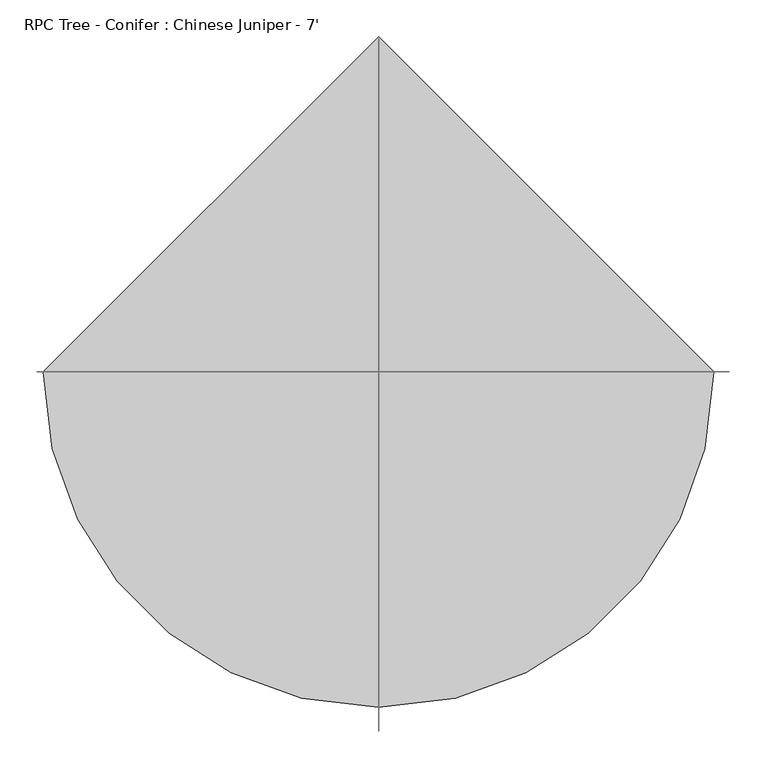
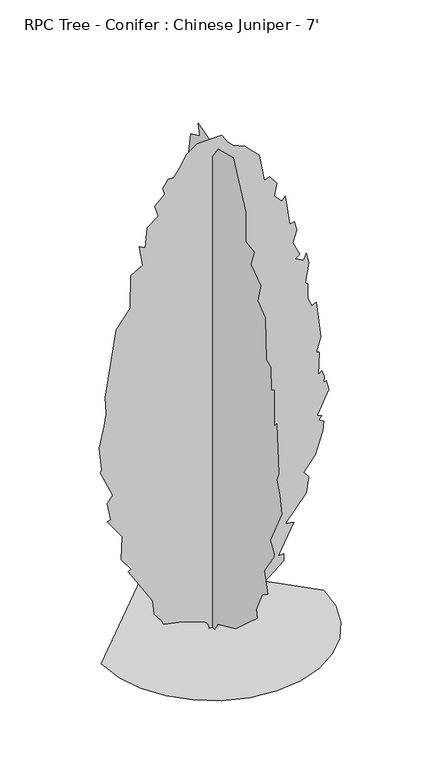
"""IFC4 building model written with IfcOpenShell, lengths in millimetres: geographic element geometry, RPC Tree - Conifer : Chinese Juniper - 7'."""

from ifc_helpers import new_model, si_unit, origin, place, context, project, spatial, triangles, source, transform, mapped, element, save


def rpc_tree_conifer_chinese_juniper_7_1b9786cd(model_context):
    return source(origin(), model_context, "Body", "Tessellation", [
        triangles([(-14.517647, 6e-07, 1.3e-06), (-18.0071097, -3e-07, 17.9396969), (-27.4223632, -6e-07, 30.3914521), (-123.5685295, 1.5e-06, 65.7757953), (-201.676062, 3.9e-06, 82.3498608), (-209.1624873, 3.1e-06, 101.0656516), (-239.326362, 2.1e-06, 139.6788561), (-246.5945957, -1e-06, 198.3880905), (-257.8249785, -1.9e-06, 220.8470939), (-347.6599566, -6.4e-06, 363.0865585), (-336.0369015, -7.4e-06, 370.071561), (-375.7854927, -8.9e-06, 425.7942498), (-371.7570322, -1.5e-05, 524.6285151), (-433.7535387, -1.74e-05, 610.1379032), (-418.7802157, -1.83e-05, 613.8793173), (-433.1718882, -2.22e-05, 689.5207758), (-411.2922644, -2.49e-05, 718.6876728), (-463.6977139, -2.95e-05, 834.7279736), (-456.2123059, -3.02e-05, 842.2133451), (-467.4416714, -3.58e-05, 943.2777431), (-447.126705, -4.19e-05, 1031.4541197), (-437.4949891, -4.53e-05, 1081.7767748), (-441.2389466, -4.94e-05, 1152.8969976), (-396.3214485, -6.81e-05, 1433.6338589), (-340.174585, -7.5e-05, 1508.4981846), (-337.1392688, -8.35e-05, 1648.2265743), (-287.7691355, -8.74e-05, 1676.941246), (-302.7424948, -9.18e-05, 1763.0323574), (-277.1874594, -9.21e-05, 1748.371479), (-269.0543621, -9.76e-05, 1834.1525803), (-224.1350836, -0.0001015, 1867.8406403), (-239.107916, -0.0001038, 1916.5022049), (-197.9328675, -0.0001078, 1953.9342224), (-205.4192747, -0.000109, 1980.1369835), (-182.9602713, -0.000112, 2013.8251888), (-160.5012679, -0.000113, 2013.8251888), (-134.7328734, -0.0001161, 2047.2821583), (-108.898967, -0.0001202, 2095.8470718), (-62.5486394, -0.0001241, 2127.2339642), (37.1144179, -0.0001285, 2128.801165), (60.3458442, -0.0001273, 2092.4307106), (82.8048476, -0.000127, 2069.9720524), (132.737601, -0.0001279, 2048.8239246), (191.3566519, -0.0001268, 1987.6224277), (213.8156735, -0.0001209, 1871.5845978), (236.2746769, -0.0001223, 1879.070042), (263.6666277, -0.0001212, 1839.8828991), (254.989959, -0.0001178, 1789.2351185), (284.9366594, -0.0001171, 1755.5469131), (299.9074571, -0.0001186, 1770.5202724), (318.6248102, -0.0001119, 1643.2505699), (337.3395836, -0.0001129, 1646.9946728), (347.517378, -0.0001111, 1609.9130699), (330.7888933, -0.0001074, 1559.0291119), (359.7983145, -0.000105, 1497.2687828), (340.1843954, -0.0001034, 1485.5084541), (374.7716738, -0.0001038, 1467.3220642), (386.0010392, -0.0001059, 1493.5248253), (397.230441, -0.0001037, 1448.6072182), (382.2596251, -9.81e-05, 1366.2577389), (393.0673594, -9.81e-05, 1357.3651131), (391.5662155, -9.44e-05, 1296.562429), (408.4598064, -9.28e-05, 1257.7053532), (427.1771233, -9.41e-05, 1265.1907974), (445.8918966, -8.55e-05, 1107.9794632), (427.1771233, -8.11e-05, 1048.0886421), (438.8332068, -8.14e-05, 1044.1287821), (434.6625312, -7.54e-05, 947.0217007), (449.6358905, -7.68e-05, 958.2511024), (460.8652559, -7.57e-05, 932.0483414), (457.1212984, -7.4e-05, 905.8481964), (468.3506639, -7.47e-05, 909.5896105), (479.5800293, -7.27e-05, 868.4161062), (430.9185737, -6.48e-05, 771.0931223), (449.6358905, -6.52e-05, 763.6077507), (438.4064887, -6.38e-05, 748.6343914), (457.1212984, -6.39e-05, 737.4049896), (453.1842567, -6.13e-05, 697.0620306), (423.4331657, -5.44e-05, 602.6499518), (374.7716738, -4.87e-05, 542.7590944), (397.230441, -4.81e-05, 516.5563697), (384.9545551, -4.37e-05, 451.166393), (299.9074571, -3.36e-05, 344.3717488), (333.5981332, -3.49e-05, 340.6277913), (269.9633001, -2.47e-05, 217.1038994), (292.4220673, -2.57e-05, 217.1038994), (292.4220673, -2.39e-05, 187.1584707), (127.7223548, -8.7e-06, 52.4044321), (127.7223548, -9.8e-06, 71.1202274), (15.4277284, -7e-07, 0.0), (0.1966721, 13.7891713, 0.00013), (0.1966737, 34.4811189, 14.2963339), (0.1966762, 77.4229995, 29.9456808), (0.1966783, 178.488651, 67.3772736), (0.1966827, 230.8930831, 116.0384931), (0.1966819, 208.4340797, 119.7817057), (0.1966904, 288.5449239, 235.2565704), (0.1966918, 264.5824875, 291.9663175), (0.196695, 331.9587347, 389.2892833), (0.1966967, 324.4733268, 434.2067814), (0.1967014, 373.1322753, 494.0976388), (0.1967052, 389.4924685, 565.7309481), (0.1967041, 380.6202267, 640.0820784), (0.1967106, 440.5110841, 729.9170746), (0.1967147, 444.2524981, 819.7546143), (0.196717, 422.6319428, 893.2725832), (0.1967196, 455.4818636, 1010.6565519), (0.19672, 425.5377248, 1051.8300562), (0.1967236, 388.1056346, 1171.611771), (0.1967244, 414.3083593, 1253.9613956), (0.1967283, 384.3616407, 1373.7430378), (0.1967298, 346.932094, 1444.8632607), (0.1967315, 328.2147772, 1594.5917667), (0.19673, 305.75601, 1583.362365), (0.1967359, 305.75601, 1718.1148956), (0.1967344, 260.8385118, 1729.3441521), (0.1967329, 237.0752094, 1809.303661), (0.1967352, 223.406676, 1875.3287006), (0.1967352, 178.488651, 1920.2461624), (0.1967401, 156.0296476, 2055.0011639), (0.1967346, 92.3955867, 2084.9454117), (0.1967371, 102.0598133, 2133.1292439), (0.1967319, 11.3487565, 2104.2112415), (0.1967329, 6.3027505, 2040.0278046), (0.1967297, -38.6152347, 2103.6627285), (0.1967262, -147.1670527, 2133.606831), (0.1967183, -237.0033388, 1950.1902649), (0.1967127, -237.0033388, 1822.9231785), (0.1967097, -296.2055936, 1812.3847229), (0.1967078, -270.691199, 1744.3175114), (0.1967065, -342.8426634, 1695.0642677), (0.196704, -323.0966666, 1617.050425), (0.1966999, -375.4995727, 1575.8744499), (0.1966957, -382.9874877, 1396.2018414), (0.1966938, -413.5488853, 1383.1639744), (0.1966894, -416.6756204, 1283.9081142), (0.196689, -439.1343876, 1298.8788574), (0.1966862, -439.1343876, 1141.6675959), (0.1966823, -457.849161, 1164.1263994), (0.1966765, -472.8225203, 954.5096884), (0.1966757, -456.5690065, 918.855542), (0.1966723, -480.3104716, 864.672076), (0.1966725, -491.5398371, 789.8078957), (0.1966689, -412.9316628, 628.8526766), (0.1966658, -439.1343876, 583.9351785), (0.1966692, -436.9195155, 568.0778978), (0.1966679, -368.0141647, 467.8974212), (0.1966629, -394.2168895, 381.8038754), (0.1966636, -353.0408054, 355.6011506), (0.1966655, -311.8672648, 265.7661362), (0.1966637, -319.3526728, 232.0767318), (0.196664, -244.4894916, 164.6997216), (0.1966643, -165.8828434, 93.5794897), (0.1966675, -34.8715179, 33.6886368), (0.1966708, -16.1562041, 0.0001282), (-457.9674314, 0.0, 0.0001492), (-445.8541446, -104.9808196, 0.0001424), (-411.358285, -201.3891246, 0.0001352), (-357.2408761, -286.4621113, 0.0001277), (-286.2654482, -357.4375574, 0.0001204), (-201.1924614, -411.5549664, 0.0001134), (-104.7841473, -446.0508259, 0.0001072), (0.1966917, -458.1641127, 0.0001019), (105.1774918, -446.0508259, 9.8e-05), (201.5857877, -411.5549664, 9.58e-05), (286.6587745, -357.4375574, 9.54e-05), (357.6342387, -286.4621113, 9.65e-05), (411.7516477, -201.3888702, 9.92e-05), (446.2475072, -104.9808196, 0.0001034), (458.360794, 4.01e-05, 0.0001092), (0.1966112, 458.1641127, 0.0001565)], [[57, 58, 59], [27, 28, 29], [87, 88, 89], [49, 50, 51], [13, 14, 15], [83, 84, 85], [74, 75, 76], [63, 64, 65], [68, 69, 70], [71, 72, 73], [9, 10, 11], [85, 86, 87], [85, 87, 89], [51, 52, 53], [54, 55, 56], [90, 1, 2], [66, 67, 68], [45, 46, 47], [17, 18, 19], [68, 70, 71], [45, 47, 48], [31, 32, 33], [76, 77, 78], [89, 90, 2], [89, 2, 3], [57, 59, 60], [51, 53, 54], [25, 26, 27], [39, 40, 41], [56, 57, 60], [71, 73, 74], [34, 35, 36], [33, 34, 36], [4, 5, 6], [60, 61, 62], [80, 81, 82], [38, 39, 41], [37, 38, 41], [37, 41, 42], [29, 30, 31], [15, 16, 17], [36, 37, 42], [33, 36, 42], [31, 33, 42], [31, 42, 43], [31, 43, 44], [31, 44, 45], [29, 31, 45], [29, 45, 48], [27, 29, 48], [25, 27, 48], [25, 48, 49], [25, 49, 51], [25, 51, 54], [25, 54, 56], [25, 56, 60], [25, 60, 62], [24, 25, 62], [23, 24, 62], [22, 23, 62], [22, 62, 63], [22, 63, 65], [22, 65, 66], [22, 66, 68], [21, 22, 68], [20, 21, 68], [19, 20, 68], [17, 19, 68], [17, 68, 71], [17, 71, 74], [15, 17, 74], [13, 15, 74], [13, 74, 76], [13, 76, 78], [13, 78, 79], [13, 79, 80], [12, 13, 80], [11, 12, 80], [9, 11, 80], [9, 80, 82], [9, 82, 83], [9, 83, 85], [9, 85, 89], [9, 89, 3], [9, 3, 4], [8, 9, 4], [8, 4, 6], [7, 8, 6], [138, 139, 140], [94, 95, 96], [136, 137, 138], [121, 122, 123], [112, 113, 114], [128, 129, 130], [121, 123, 124], [125, 126, 127], [124, 125, 127], [114, 115, 116], [147, 148, 149], [130, 131, 132], [124, 127, 128], [134, 135, 136], [154, 155, 91], [154, 91, 92], [150, 151, 152], [96, 97, 98], [119, 120, 121], [119, 121, 124], [119, 124, 128], [118, 119, 128], [117, 118, 128], [116, 117, 128], [116, 128, 130], [114, 116, 130], [114, 130, 132], [112, 114, 132], [112, 132, 133], [112, 133, 134], [112, 134, 136], [111, 112, 136], [110, 111, 136], [109, 110, 136], [109, 136, 138], [109, 138, 140], [109, 140, 141], [108, 109, 141], [107, 108, 141], [106, 107, 141], [105, 106, 141], [104, 105, 141], [103, 104, 141], [103, 141, 142], [103, 142, 143], [103, 143, 144], [102, 103, 144], [101, 102, 144], [100, 101, 144], [100, 144, 145], [100, 145, 146], [100, 146, 147], [100, 147, 149], [100, 149, 150], [100, 150, 152], [100, 152, 153], [100, 153, 154], [99, 100, 154], [98, 99, 154], [96, 98, 154], [96, 154, 92], [96, 92, 93], [96, 93, 94], [170, 171, 156], [169, 170, 156], [169, 156, 157], [168, 169, 157], [168, 157, 158], [168, 158, 159], [167, 168, 159], [166, 167, 159], [166, 159, 160], [166, 160, 161], [166, 161, 162], [166, 162, 163], [166, 163, 164], [166, 164, 165]], closed=False),
    ])


if __name__ == "__main__":
    model = new_model("IFC4")
    model_context = context("Model", 3, world=origin())
    ifc_project = project(units=[si_unit("LENGTHUNIT", "METRE", prefix="MILLI")], contexts=[model_context])
    site = spatial("IfcSite", under=ifc_project)
    building = spatial("IfcBuilding", under=site)
    placement = place(None, origin())
    rpc_tree_conifer_chinese_juniper_7_shape = rpc_tree_conifer_chinese_juniper_7_1b9786cd(model_context)
    element("IfcGeographicElement", 1, ObjectType="RPC Tree - Conifer : Chinese Juniper - 7'", at=placement, inside=building, context=model_context, shape_type="MappedRepresentation", body=[
        mapped(rpc_tree_conifer_chinese_juniper_7_shape, transform((0.0, 0.0, 0.0), x_axis=(1.0, 0.0, 0.0), y_axis=(0.0, 1.0, 0.0), z_axis=(0.0, 0.0, 1.0))),
    ])
    save(model, "model.ifc")

# Revit data of these elements
# Type "RPC Tree - Conifer : Chinese Juniper - 7'"
#   built-in parameter 1005198 = "{2, 15},{39, RPC-16-FUM3-UUQ0-UBF0-N000-ST1L-LVER-AU},{1, 0},{1, 0},{2, 13},{1, 8},{5, Color},{1, 0},{1, 0},{3, 0.8},{3, 0.8},{3, 0.8},{1, 8},{7, BBoxMin},{1, 0},{1, 0},{1, 0},{1, 0},{1, 0},{1, 8},{7, BBoxMax},{1, 0},{1, 0},{1, 0},{1, 0},{1, 0},{2, 11},{9, RPCTypeId},{1, 0},{1, 0},{39, RPC-16-FUM3-UUQ0-UBF0-N000-ST1L-LVER-AU},{1, 6},{14, RPCPlantHeight},{1, 0},{1, 0},{1, 7},{2, 11},{7, keyword},{1, 0},{1, 0},{34, :RPCs:Trees [General]:Geometry:RPC},{2, 11},{8, category},{1, 0},{1, 0},{15, Trees [General]},{2, 11},{12, LocalizedUID},{1, 0},{1, 0},{15, Chinese Juniper},{2, 14},{6, Height},{1, 0},{1, 0},{1, 7},{1, 2},{16, Cast Reflections},{1, 0},{1, 0},{1, 0},{1, 2},{12, Cast Shadows},{1, 0},{1, 0},{1, 1},{1, 2},{9, Lock View},{1, 0},{1, 0},{1, 0},{1, 4},{5, ViewC},{1, 0},{1, 0},{1, 0},{21, assetlibrary_base.fbx},{1, 5},"
#   built-in parameter 1005195 = "RPC-16-FUM3-UUQ0-UBF0-N000-ST1L-LVER-AU"
#   Type Comments = "Chinese Juniper"
#   Assembly Code = "G2050500"
#   Height = 7' - 0"
#   Description = (empty or 0)
#   Default Elevation = 0
